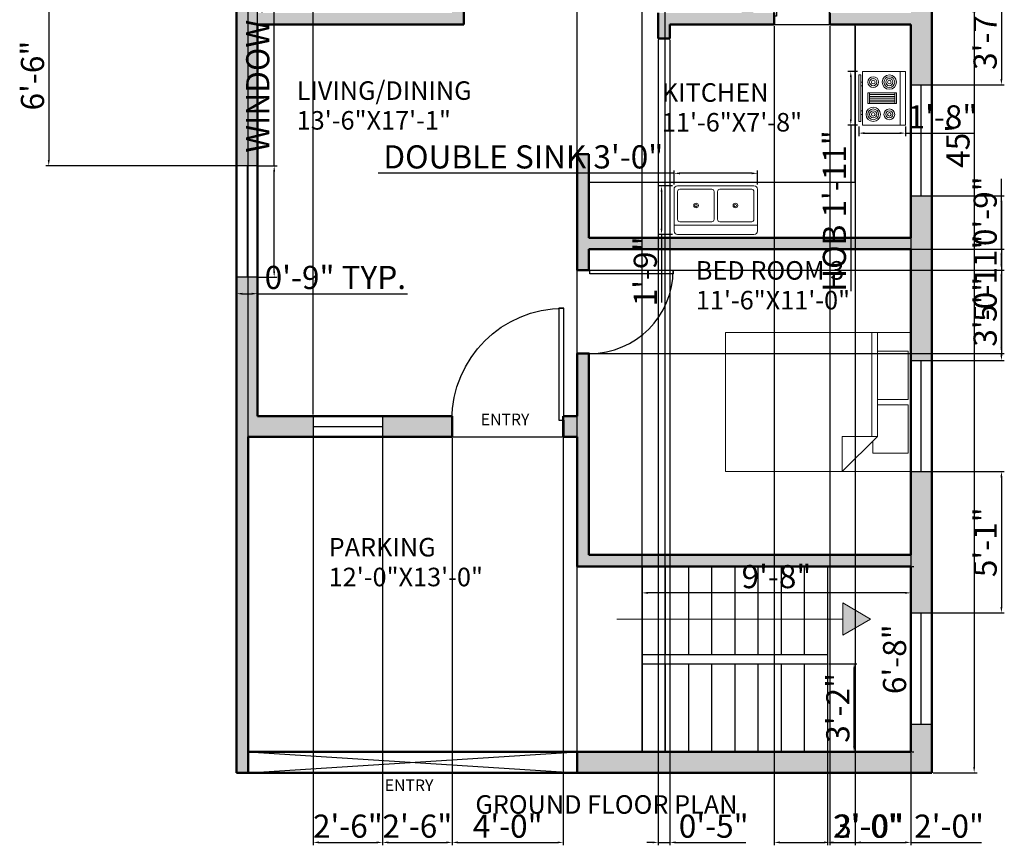
# Model space of a CAD drawing. Units: inches. Extents: x 3560 to 3985, y 1331 to 2044.
# Tile 1 of 2: x 3560 to 3985, y 1331 to 1688. Entities that reach past the tile are written whole.
import ezdxf

# ---------------------------------------------------------------- set-up
doc = ezdxf.new("R2010")
doc.units = ezdxf.units.IN
for name, color, linetype, lineweight in [('A-ANNO-DIMS', 5, 'Continuous', 18), ('A-ANNO-SYMB', 3, 'Continuous', 18), ('A-ANNO-TEXT', 2, 'Continuous', 25), ('A-AREA-IDEN', 3, 'Continuous', 25), ('A-EQPM', 8, 'Continuous', 18), ('A-FLOR-CASE', 8, 'Continuous', 25), ('A-FLOR-FIXT', 9, 'Continuous', 18), ('A-FURN', 8, 'Continuous', 18), ('A-WALL-PATT', 7, 'Continuous', 13), ('DOOR', 6, 'Continuous', 25), ('STAIRS', 1, 'Continuous', 25), ('WALL', 52, 'Continuous', 50), ('WINDOW', 4, 'Continuous', 25)]:
    doc.layers.add(name, color=color, linetype=linetype, lineweight=lineweight)
doc.styles.get("Standard").update_dxf_attribs({"font": 'arial.ttf'})
doc.dimstyles.new('ISO-25', dxfattribs={"dimtxt": 10, "dimasz": 2.5, "dimexe": 1.25, "dimexo": 0.625, "dimtad": 1, "dimdec": 1, "dimlunit": 3, "dimtxsty": 'Standard', "dimcen": 2.5, "dimadec": 0, "dimazin": 0, "dimtfac": 1, "dimtdec": 1, "dimtmove": 0, "dimatfit": 3, "dimfxl": 1, "dimarcsym": 0})

# ---------------------------------------------------------------- blocks, each defined once
blk = doc.blocks.new('*D1')
at = {"layer": 'A-ANNO-DIMS', "color": 0, "lineweight": -2, "transparency": 16777216}
for p, q in [((3828.42, 1450.94), (3828.42, 1438.95)), ((3944.42, 1450.94), (3944.42, 1438.95)), ((3941.92, 1440.2), (3830.92, 1440.2))]:
    blk.add_line(p, q, dxfattribs=at)
at = {"layer": 'A-ANNO-DIMS', "color": 0, "transparency": 16777216}
for points in [[(3830.92, 1440.62), (3830.92, 1439.78), (3828.42, 1440.2)], [(3941.92, 1440.62), (3941.92, 1439.78), (3944.42, 1440.2)]]:
    blk.add_solid(points, dxfattribs=at)
at = {"layer": 'Defpoints', "color": 0, "transparency": 16777216}
for p in [(3828.42, 1451.56), (3944.42, 1451.56), (3828.42, 1440.2)]:
    blk.add_point(p, dxfattribs=at)
at = {"layer": 'A-ANNO-DIMS', "color": 0, "transparency": 16777216, "insert": (3886.42, 1445.93), "char_height": 10, "attachment_point": 5}
blk.add_mtext('9\'-8"', dxfattribs=at)
blk = doc.blocks.new('*D2')
at = {"layer": 'A-ANNO-DIMS', "color": 0, "lineweight": -2, "transparency": 16777216}
for p, q in [((3945.04, 1451.56), (3945.67, 1451.56)), ((3944.42, 1449.06), (3944.42, 1374.06)), ((3945.04, 1371.56), (3945.67, 1371.56))]:
    blk.add_line(p, q, dxfattribs=at)
at = {"layer": 'A-ANNO-DIMS', "color": 0, "transparency": 16777216}
for points in [[(3944, 1449.06), (3944.83, 1449.06), (3944.42, 1451.56)], [(3944, 1374.06), (3944.83, 1374.06), (3944.42, 1371.56)]]:
    blk.add_solid(points, dxfattribs=at)
at = {"layer": 'Defpoints', "color": 0, "transparency": 16777216}
for p in [(3944.42, 1451.56), (3944.42, 1371.56), (3944.42, 1371.56)]:
    blk.add_point(p, dxfattribs=at)
at = {"layer": 'A-ANNO-DIMS', "color": 0, "transparency": 16777216, "insert": (3938.69, 1411.56), "char_height": 10, "attachment_point": 5, "rotation": 90}
blk.add_mtext('6\'-8"', dxfattribs=at)
blk = doc.blocks.new('*D3')
at = {"layer": 'A-ANNO-DIMS', "color": 0, "lineweight": -2, "transparency": 16777216}
for p, q in [((3909.04, 1409.56), (3921.18, 1409.56)), ((3919.93, 1374.06), (3919.93, 1407.06)), ((3909.04, 1371.56), (3921.18, 1371.56))]:
    blk.add_line(p, q, dxfattribs=at)
at = {"layer": 'A-ANNO-DIMS', "color": 0, "transparency": 16777216}
for points in [[(3919.52, 1407.06), (3920.35, 1407.06), (3919.93, 1409.56)], [(3919.52, 1374.06), (3920.35, 1374.06), (3919.93, 1371.56)]]:
    blk.add_solid(points, dxfattribs=at)
at = {"layer": 'Defpoints', "color": 0, "transparency": 16777216}
for p in [(3908.42, 1409.56), (3919.93, 1409.56), (3908.42, 1371.56)]:
    blk.add_point(p, dxfattribs=at)
at = {"layer": 'A-ANNO-DIMS', "color": 0, "transparency": 16777216, "insert": (3914.2, 1390.56), "char_height": 10, "attachment_point": 5, "rotation": 90}
blk.add_mtext('3\'-2"', dxfattribs=at)
blk = doc.blocks.new('*U5')
for p, q in [((0, 0), (0, -6)), ((40, 0), (40, -6))]:
    blk.add_line(p, q)
blk.add_lwpolyline([(0, 0), (0, 40), (1.75, 40), (1.75, 0)], close=True)
blk.add_arc((0, 0), 40, 0, 90)
blk = doc.blocks.new('Range-Oven - 30 in top')
for p, q in [((0, -3), (30, -3)), ((12, -6), (18, -6)), ((13, -20), (13, -6)), ((14, -6), (14, -20)), ((15, -20), (15, -6)), ((16, -6), (16, -20)), ((17, -20), (17, -6)), ((18, -20), (12, -20)), ((6, -24), (6, -25)), ((8, -25), (8, -24)), ((22, -25), (22, -24)), ((24, -24), (24, -25))]:
    blk.add_line(p, q)
for points in [[(0, -24), (0, 0), (30, 0), (30, -24)], [(12, -21), (12, -5), (18, -5), (18, -21)], [(2, -26), (2, -25), (28, -25), (28, -26)]]:
    blk.add_lwpolyline(points, close=True)
for centre, radius in [((6, -9), 4), ((6, -9), 3), ((6, -9), 2), ((6, -9), 1), ((24, -9), 3), ((24, -9), 2), ((24, -9), 1), ((6, -18), 3), ((6, -18), 2), ((24, -18), 4), ((24, -18), 3), ((24, -18), 2), ((6, -18), 1), ((24, -18), 1)]:
    blk.add_circle(centre, radius)
blk = doc.blocks.new('Sink-double - 36 in top')
for p, q in [((-18, -4), (18, -4)), ((-0.75, -18.5), (-0.75, -6.5)), ((0.75, -6.5), (0.75, -18.5))]:
    blk.add_line(p, q)
for points in [[(-16.5, 0), (16.5, 0)], [(-18, -19.5), (-18, -1.5)], [(18, -1.5), (18, -19.5)], [(-16.5, -18.5), (-16.5, -6.5)], [(-15.5, -5.5), (-1.75, -5.5)], [(1.75, -5.5), (15.5, -5.5)], [(16.5, -6.5), (16.5, -18.5)], [(16.5, -21), (-16.5, -21)], [(-1.75, -19.5), (-15.5, -19.5)], [(15.5, -19.5), (1.75, -19.5)]]:
    blk.add_lwpolyline(points)
for centre, radius in [((-8.5, -12.5), 1), ((-8.5, -12.5), 0.5), ((8.5, -12.5), 1), ((8.5, -12.5), 0.5)]:
    blk.add_circle(centre, radius)
for centre, radius, start, end in [((-16.5, -1.5), 1.5, 90, 180), ((16.5, -1.5), 1.5, 0, 90), ((-15.5, -6.5), 1, 90, 180), ((-1.75, -6.5), 1, 0, 90), ((1.75, -6.5), 1, 90, 180), ((15.5, -6.5), 1, 0, 90), ((-16.5, -19.5), 1.5, 180, 270), ((-15.5, -18.5), 1, 180, 270), ((-1.75, -18.5), 1, 270, 0), ((1.75, -18.5), 1, 180, 270), ((15.5, -18.5), 1, 270, 0), ((16.5, -19.5), 1.5, 270, 0)]:
    blk.add_arc(centre, radius, start, end)
blk = doc.blocks.new('Bed - Queen')
for p, q in [((0, -80.00003), (0, 0)), ((0, 0), (59.99999, 0)), ((59.99999, 0), (59.99999, -80.00003)), ((7.99999, -1.2), (28.79998, -1.2)), ((7.99999, -14.4), (7.99999, -1.2)), ((28.79998, -1.2), (28.79998, -14.4)), ((31.19999, -1.2), (51.99999, -1.2)), ((31.19999, -14.4), (31.19999, -1.2)), ((51.99999, -1.2), (51.99999, -16.4)), ((0, -14.4), (44.8, -14.4)), ((44.8, -16.8), (0, -16.8)), ((59.99999, -29.6), (44.8, -14.4)), ((44.8, -14.4), (44.8, -29.6)), ((51.99999, -16.4), (46.79936, -16.4)), ((44.8, -29.6), (59.99999, -29.6)), ((59.99999, -80.00003), (0, -80.00003))]:
    blk.add_line(p, q)
blk = doc.blocks.new('*D12')
at = {"layer": 'A-ANNO-DIMS', "color": 0, "lineweight": -2, "transparency": 16777216}
for p, q in [((3954.04, 1902.56), (3973, 1902.56)), ((3971.75, 1900.06), (3971.75, 1365.06)), ((3954.04, 1362.56), (3973, 1362.56))]:
    blk.add_line(p, q, dxfattribs=at)
at = {"layer": 'A-ANNO-DIMS', "color": 0, "transparency": 16777216}
for points in [[(3971.33, 1900.06), (3972.16, 1900.06), (3971.75, 1902.56)], [(3971.33, 1365.06), (3972.16, 1365.06), (3971.75, 1362.56)]]:
    blk.add_solid(points, dxfattribs=at)
at = {"layer": 'Defpoints', "color": 0, "transparency": 16777216}
for p in [(3953.42, 1902.56), (3953.42, 1362.56), (3971.75, 1362.56)]:
    blk.add_point(p, dxfattribs=at)
at = {"layer": 'A-ANNO-DIMS', "color": 0, "transparency": 16777216, "insert": (3966.04, 1633.18), "char_height": 10, "attachment_point": 5, "rotation": 90}
blk.add_mtext("45'", dxfattribs=at)
blk = doc.blocks.new('WIN-48IN')
for p, q in [((9, 48), (0, 48)), ((4.5, 48), (4.5, 0)), ((9, 0), (0, 0))]:
    blk.add_line(p, q)
blk = doc.blocks.new('*D20')
at = {"layer": 'A-ANNO-DIMS', "color": 0, "lineweight": -2, "transparency": 16777216}
for p, q in [((3669.62, 1624.56), (3669.62, 1754.85)), ((3663.04, 1624.56), (3670.87, 1624.56)), ((3669.62, 1579.06), (3669.62, 1622.06)), ((3663.04, 1576.56), (3670.87, 1576.56))]:
    blk.add_line(p, q, dxfattribs=at)
at = {"layer": 'A-ANNO-DIMS', "color": 0, "transparency": 16777216}
for points in [[(3669.2, 1622.06), (3670.03, 1622.06), (3669.62, 1624.56)], [(3669.2, 1579.06), (3670.03, 1579.06), (3669.62, 1576.56)]]:
    blk.add_solid(points, dxfattribs=at)
at = {"layer": 'Defpoints', "color": 0, "transparency": 16777216}
for p in [(3662.42, 1624.56), (3669.62, 1624.56), (3662.42, 1576.56)]:
    blk.add_point(p, dxfattribs=at)
at = {"layer": 'A-ANNO-DIMS', "color": 0, "transparency": 16777216, "insert": (3663.82, 1690.96), "char_height": 10, "attachment_point": 5, "rotation": 90}
blk.add_mtext('WINDOW 4\'-0" TYP.', dxfattribs=at)
blk = doc.blocks.new('*D21')
at = {"layer": 'A-ANNO-DIMS', "color": 0, "lineweight": -2, "transparency": 16777216}
for p, q in [((3653.42, 1575.94), (3653.42, 1568.11)), ((3662.42, 1575.94), (3662.42, 1568.11)), ((3655.92, 1569.36), (3659.92, 1569.36)), ((3662.42, 1569.36), (3727.12, 1569.36))]:
    blk.add_line(p, q, dxfattribs=at)
at = {"layer": 'A-ANNO-DIMS', "color": 0, "transparency": 16777216}
for points in [[(3655.92, 1569.78), (3655.92, 1568.95), (3653.42, 1569.36)], [(3659.92, 1569.78), (3659.92, 1568.95), (3662.42, 1569.36)]]:
    blk.add_solid(points, dxfattribs=at)
at = {"layer": 'Defpoints', "color": 0, "transparency": 16777216}
for p in [(3653.42, 1576.56), (3662.42, 1576.56), (3662.42, 1569.36)]:
    blk.add_point(p, dxfattribs=at)
at = {"layer": 'A-ANNO-DIMS', "color": 0, "transparency": 16777216, "insert": (3696.02, 1575.09), "char_height": 10, "attachment_point": 5}
blk.add_mtext('0\'-9" TYP.', dxfattribs=at)
blk = doc.blocks.new('*D24')
at = {"layer": 'A-ANNO-DIMS', "color": 0, "lineweight": -2, "transparency": 16777216}
for p, q in [((3921.37, 1665.36), (3917.26, 1665.36)), ((3918.51, 1662.86), (3918.51, 1644.66)), ((3921.37, 1642.16), (3917.26, 1642.16)), ((3918.51, 1642.16), (3918.51, 1570.44))]:
    blk.add_line(p, q, dxfattribs=at)
at = {"layer": 'A-ANNO-DIMS', "color": 0, "transparency": 16777216}
for points in [[(3918.1, 1662.86), (3918.93, 1662.86), (3918.51, 1665.36)], [(3918.1, 1644.66), (3918.93, 1644.66), (3918.51, 1642.16)]]:
    blk.add_solid(points, dxfattribs=at)
at = {"layer": 'Defpoints', "color": 0, "transparency": 16777216}
for p in [(3921.99, 1665.36), (3918.51, 1642.16), (3921.99, 1642.16)]:
    blk.add_point(p, dxfattribs=at)
at = {"layer": 'A-ANNO-DIMS', "color": 0, "transparency": 16777216, "insert": (3912.72, 1605.05), "char_height": 10, "attachment_point": 5, "rotation": 90}
blk.add_mtext('HOB 1\'-11"', dxfattribs=at)
blk = doc.blocks.new('*D25')
at = {"layer": 'A-ANNO-DIMS', "color": 0, "lineweight": -2, "transparency": 16777216}
for p, q in [((3921.99, 1641.54), (3921.99, 1637.43)), ((3942.1, 1641.54), (3942.1, 1637.43)), ((3924.49, 1638.68), (3939.6, 1638.68)), ((3942.1, 1638.68), (3971.49, 1638.68))]:
    blk.add_line(p, q, dxfattribs=at)
at = {"layer": 'A-ANNO-DIMS', "color": 0, "transparency": 16777216}
for points in [[(3924.49, 1639.1), (3924.49, 1638.26), (3921.99, 1638.68)], [(3939.6, 1639.1), (3939.6, 1638.26), (3942.1, 1638.68)]]:
    blk.add_solid(points, dxfattribs=at)
at = {"layer": 'Defpoints', "color": 0, "transparency": 16777216}
for p in [(3921.99, 1642.16), (3942.1, 1642.16), (3942.1, 1638.68)]:
    blk.add_point(p, dxfattribs=at)
at = {"layer": 'A-ANNO-DIMS', "color": 0, "transparency": 16777216, "insert": (3958.04, 1644.41), "char_height": 10, "attachment_point": 5}
blk.add_mtext('1\'-8"', dxfattribs=at)
blk = doc.blocks.new('*D26')
at = {"layer": 'A-ANNO-DIMS', "color": 0, "lineweight": -2, "transparency": 16777216}
for p, q in [((3842.22, 1621.34), (3714.57, 1621.34)), ((3842.22, 1616.56), (3842.22, 1622.59)), ((3875.72, 1621.34), (3844.72, 1621.34)), ((3878.22, 1616.56), (3878.22, 1622.59))]:
    blk.add_line(p, q, dxfattribs=at)
at = {"layer": 'A-ANNO-DIMS', "color": 0, "transparency": 16777216}
for points in [[(3844.72, 1621.75), (3844.72, 1620.92), (3842.22, 1621.34)], [(3875.72, 1621.75), (3875.72, 1620.92), (3878.22, 1621.34)]]:
    blk.add_solid(points, dxfattribs=at)
at = {"layer": 'Defpoints', "color": 0, "transparency": 16777216}
for p in [(3842.22, 1621.34), (3842.22, 1615.94), (3878.22, 1615.94)]:
    blk.add_point(p, dxfattribs=at)
at = {"layer": 'A-ANNO-DIMS', "color": 0, "transparency": 16777216, "insert": (3777.15, 1627.14), "char_height": 10, "attachment_point": 5}
blk.add_mtext('DOUBLE SINK 3\'-0"', dxfattribs=at)
blk = doc.blocks.new('*D27')
at = {"layer": 'A-ANNO-DIMS', "color": 0, "lineweight": -2, "transparency": 16777216}
for p, q in [((3841.6, 1615.94), (3835.57, 1615.94)), ((3836.82, 1613.44), (3836.82, 1597.44)), ((3841.6, 1594.94), (3835.57, 1594.94)), ((3836.82, 1594.94), (3836.82, 1565.54))]:
    blk.add_line(p, q, dxfattribs=at)
at = {"layer": 'A-ANNO-DIMS', "color": 0, "transparency": 16777216}
for points in [[(3836.41, 1613.44), (3837.24, 1613.44), (3836.82, 1615.94)], [(3836.41, 1597.44), (3837.24, 1597.44), (3836.82, 1594.94)]]:
    blk.add_solid(points, dxfattribs=at)
at = {"layer": 'Defpoints', "color": 0, "transparency": 16777216}
for p in [(3842.22, 1615.94), (3836.82, 1594.94), (3842.22, 1594.94)]:
    blk.add_point(p, dxfattribs=at)
at = {"layer": 'A-ANNO-DIMS', "color": 0, "transparency": 16777216, "insert": (3831.09, 1578.99), "char_height": 10, "attachment_point": 5, "rotation": 90}
blk.add_mtext('1\'-9"', dxfattribs=at)
blk = doc.blocks.new('*D30')
at = {"layer": 'A-ANNO-DIMS', "color": 0, "lineweight": -2, "transparency": 16777216}
for p, q in [((3652.79, 1702.56), (3571.07, 1702.56)), ((3572.32, 1700.06), (3572.32, 1627.06)), ((3652.79, 1624.56), (3571.07, 1624.56))]:
    blk.add_line(p, q, dxfattribs=at)
at = {"layer": 'A-ANNO-DIMS', "color": 0, "transparency": 16777216}
for points in [[(3571.9, 1700.06), (3572.73, 1700.06), (3572.32, 1702.56)], [(3571.9, 1627.06), (3572.73, 1627.06), (3572.32, 1624.56)]]:
    blk.add_solid(points, dxfattribs=at)
at = {"layer": 'Defpoints', "color": 0, "transparency": 16777216}
for p in [(3653.42, 1702.56), (3572.32, 1624.56), (3653.42, 1624.56)]:
    blk.add_point(p, dxfattribs=at)
at = {"layer": 'A-ANNO-DIMS', "color": 0, "transparency": 16777216, "insert": (3566.59, 1663.56), "char_height": 10, "attachment_point": 5, "rotation": 90}
blk.add_mtext('6\'-6"', dxfattribs=at)
blk = doc.blocks.new('*D33')
at = {"layer": 'A-ANNO-DIMS', "color": 0, "lineweight": -2, "transparency": 16777216}
for p, q in [((3954.04, 1702.56), (3984.77, 1702.56)), ((3983.52, 1700.06), (3983.52, 1662.06)), ((3954.04, 1659.56), (3984.77, 1659.56))]:
    blk.add_line(p, q, dxfattribs=at)
at = {"layer": 'A-ANNO-DIMS', "color": 0, "transparency": 16777216}
for points in [[(3983.1, 1700.06), (3983.93, 1700.06), (3983.52, 1702.56)], [(3983.1, 1662.06), (3983.93, 1662.06), (3983.52, 1659.56)]]:
    blk.add_solid(points, dxfattribs=at)
at = {"layer": 'Defpoints', "color": 0, "transparency": 16777216}
for p in [(3953.42, 1702.56), (3953.42, 1659.56), (3983.52, 1659.56)]:
    blk.add_point(p, dxfattribs=at)
at = {"layer": 'A-ANNO-DIMS', "color": 0, "transparency": 16777216, "insert": (3977.78, 1681.06), "char_height": 10, "attachment_point": 5, "rotation": 90}
blk.add_mtext('3\'-7"', dxfattribs=at)
blk = doc.blocks.new('*D34')
at = {"layer": 'A-ANNO-DIMS', "color": 0, "lineweight": -2, "transparency": 16777216}
for p, q in [((3954.04, 1611.56), (3984.77, 1611.56)), ((3983.52, 1609.06), (3983.52, 1543.06)), ((3954.04, 1540.56), (3984.77, 1540.56))]:
    blk.add_line(p, q, dxfattribs=at)
at = {"layer": 'A-ANNO-DIMS', "color": 0, "transparency": 16777216}
for points in [[(3983.1, 1609.06), (3983.93, 1609.06), (3983.52, 1611.56)], [(3983.1, 1543.06), (3983.93, 1543.06), (3983.52, 1540.56)]]:
    blk.add_solid(points, dxfattribs=at)
at = {"layer": 'Defpoints', "color": 0, "transparency": 16777216}
for p in [(3953.42, 1611.56), (3953.42, 1540.56), (3983.52, 1540.56)]:
    blk.add_point(p, dxfattribs=at)
at = {"layer": 'A-ANNO-DIMS', "color": 0, "transparency": 16777216, "insert": (3977.79, 1576.06), "char_height": 10, "attachment_point": 5, "rotation": 90}
blk.add_mtext('5\'-11"', dxfattribs=at)
blk = doc.blocks.new('*D35')
at = {"layer": 'A-ANNO-DIMS', "color": 0, "lineweight": -2, "transparency": 16777216}
for p, q in [((3954.04, 1492.56), (3984.77, 1492.56)), ((3983.52, 1490.06), (3983.52, 1434.06)), ((3954.04, 1431.56), (3984.77, 1431.56))]:
    blk.add_line(p, q, dxfattribs=at)
at = {"layer": 'A-ANNO-DIMS', "color": 0, "transparency": 16777216}
for points in [[(3983.1, 1490.06), (3983.93, 1490.06), (3983.52, 1492.56)], [(3983.1, 1434.06), (3983.93, 1434.06), (3983.52, 1431.56)]]:
    blk.add_solid(points, dxfattribs=at)
at = {"layer": 'Defpoints', "color": 0, "transparency": 16777216}
for p in [(3953.42, 1492.56), (3953.42, 1431.56), (3983.52, 1431.56)]:
    blk.add_point(p, dxfattribs=at)
at = {"layer": 'A-ANNO-DIMS', "color": 0, "transparency": 16777216, "insert": (3977.79, 1462.06), "char_height": 10, "attachment_point": 5, "rotation": 90}
blk.add_mtext('5\'-1"', dxfattribs=at)
blk = doc.blocks.new('*D36')
at = {"layer": 'A-ANNO-DIMS', "color": 0, "lineweight": -2, "transparency": 16777216}
for p, q in [((3662.42, 1517.19), (3662.42, 1933.91)), ((3686.42, 1517.19), (3686.42, 1933.91)), ((3664.92, 1932.66), (3683.92, 1932.66)), ((3686.42, 1932.66), (3716.92, 1932.66))]:
    blk.add_line(p, q, dxfattribs=at)
at = {"layer": 'A-ANNO-DIMS', "color": 0, "transparency": 16777216}
for points in [[(3664.92, 1933.08), (3664.92, 1932.25), (3662.42, 1932.66)], [(3683.92, 1933.08), (3683.92, 1932.25), (3686.42, 1932.66)]]:
    blk.add_solid(points, dxfattribs=at)
at = {"layer": 'Defpoints', "color": 0, "transparency": 16777216}
for p in [(3686.42, 1932.66), (3662.42, 1516.56), (3686.42, 1516.56)]:
    blk.add_point(p, dxfattribs=at)
at = {"layer": 'A-ANNO-DIMS', "color": 0, "transparency": 16777216, "insert": (3702.92, 1938.39), "char_height": 10, "attachment_point": 5}
blk.add_mtext('2\'-0"', dxfattribs=at)
blk = doc.blocks.new('*D37')
at = {"layer": 'A-ANNO-DIMS', "color": 0, "lineweight": -2, "transparency": 16777216}
for p, q in [((3686.42, 1506.94), (3686.42, 1331.21)), ((3716.42, 1506.94), (3716.42, 1331.21)), ((3688.92, 1332.46), (3713.92, 1332.46))]:
    blk.add_line(p, q, dxfattribs=at)
at = {"layer": 'A-ANNO-DIMS', "color": 0, "transparency": 16777216}
for points in [[(3688.92, 1332.88), (3688.92, 1332.05), (3686.42, 1332.46)], [(3713.92, 1332.88), (3713.92, 1332.05), (3716.42, 1332.46)]]:
    blk.add_solid(points, dxfattribs=at)
at = {"layer": 'Defpoints', "color": 0, "transparency": 16777216}
for p in [(3686.42, 1507.56), (3716.42, 1507.56), (3716.42, 1332.46)]:
    blk.add_point(p, dxfattribs=at)
at = {"layer": 'A-ANNO-DIMS', "color": 0, "transparency": 16777216, "insert": (3701.42, 1338.19), "char_height": 10, "attachment_point": 5}
blk.add_mtext('2\'-6"', dxfattribs=at)
blk = doc.blocks.new('*D38')
at = {"layer": 'A-ANNO-DIMS', "color": 0, "lineweight": -2, "transparency": 16777216}
for p, q in [((3716.42, 1506.94), (3716.42, 1331.21)), ((3746.42, 1506.94), (3746.42, 1331.21)), ((3718.92, 1332.46), (3743.92, 1332.46))]:
    blk.add_line(p, q, dxfattribs=at)
at = {"layer": 'A-ANNO-DIMS', "color": 0, "transparency": 16777216}
for points in [[(3718.92, 1332.88), (3718.92, 1332.05), (3716.42, 1332.46)], [(3743.92, 1332.88), (3743.92, 1332.05), (3746.42, 1332.46)]]:
    blk.add_solid(points, dxfattribs=at)
at = {"layer": 'Defpoints', "color": 0, "transparency": 16777216}
for p in [(3716.42, 1507.56), (3746.42, 1507.56), (3746.42, 1332.46)]:
    blk.add_point(p, dxfattribs=at)
at = {"layer": 'A-ANNO-DIMS', "color": 0, "transparency": 16777216, "insert": (3731.42, 1338.19), "char_height": 10, "attachment_point": 5}
blk.add_mtext('2\'-6"', dxfattribs=at)
blk = doc.blocks.new('*D39')
at = {"layer": 'A-ANNO-DIMS', "color": 0, "lineweight": -2, "transparency": 16777216}
for p, q in [((3746.42, 1506.94), (3746.42, 1331.21)), ((3794.42, 1506.94), (3794.42, 1331.21)), ((3748.92, 1332.46), (3791.92, 1332.46))]:
    blk.add_line(p, q, dxfattribs=at)
at = {"layer": 'A-ANNO-DIMS', "color": 0, "transparency": 16777216}
for points in [[(3748.92, 1332.88), (3748.92, 1332.05), (3746.42, 1332.46)], [(3791.92, 1332.88), (3791.92, 1332.05), (3794.42, 1332.46)]]:
    blk.add_solid(points, dxfattribs=at)
at = {"layer": 'Defpoints', "color": 0, "transparency": 16777216}
for p in [(3746.42, 1507.56), (3794.42, 1507.56), (3794.42, 1332.46)]:
    blk.add_point(p, dxfattribs=at)
at = {"layer": 'A-ANNO-DIMS', "color": 0, "transparency": 16777216, "insert": (3770.42, 1338.19), "char_height": 10, "attachment_point": 5}
blk.add_mtext('4\'-0"', dxfattribs=at)
blk = doc.blocks.new('*D44')
at = {"layer": 'A-ANNO-DIMS', "color": 0, "lineweight": -2, "transparency": 16777216}
for p, q in [((3885.42, 1684.94), (3885.42, 1331.21)), ((3909.42, 1684.94), (3909.42, 1331.21)), ((3887.92, 1332.46), (3906.92, 1332.46)), ((3909.42, 1332.46), (3939.92, 1332.46))]:
    blk.add_line(p, q, dxfattribs=at)
at = {"layer": 'A-ANNO-DIMS', "color": 0, "transparency": 16777216}
for points in [[(3887.92, 1332.88), (3887.92, 1332.05), (3885.42, 1332.46)], [(3906.92, 1332.88), (3906.92, 1332.05), (3909.42, 1332.46)]]:
    blk.add_solid(points, dxfattribs=at)
at = {"layer": 'Defpoints', "color": 0, "transparency": 16777216}
for p in [(3885.42, 1685.56), (3909.42, 1685.56), (3909.42, 1332.46)]:
    blk.add_point(p, dxfattribs=at)
at = {"layer": 'A-ANNO-DIMS', "color": 0, "transparency": 16777216, "insert": (3925.92, 1338.19), "char_height": 10, "attachment_point": 5}
blk.add_mtext('2\'-0"', dxfattribs=at)
blk = doc.blocks.new('*D46')
at = {"layer": 'A-ANNO-DIMS', "color": 0, "lineweight": -2, "transparency": 16777216}
for p, q in [((3920.42, 1684.94), (3920.42, 1331.21)), ((3944.42, 1684.94), (3944.42, 1331.21)), ((3922.92, 1332.46), (3941.92, 1332.46)), ((3944.42, 1332.46), (3974.92, 1332.46))]:
    blk.add_line(p, q, dxfattribs=at)
at = {"layer": 'A-ANNO-DIMS', "color": 0, "transparency": 16777216}
for points in [[(3922.92, 1332.88), (3922.92, 1332.05), (3920.42, 1332.46)], [(3941.92, 1332.88), (3941.92, 1332.05), (3944.42, 1332.46)]]:
    blk.add_solid(points, dxfattribs=at)
at = {"layer": 'Defpoints', "color": 0, "transparency": 16777216}
for p in [(3920.42, 1685.56), (3944.42, 1685.56), (3944.42, 1332.46)]:
    blk.add_point(p, dxfattribs=at)
at = {"layer": 'A-ANNO-DIMS', "color": 0, "transparency": 16777216, "insert": (3960.92, 1338.19), "char_height": 10, "attachment_point": 5}
blk.add_mtext('2\'-0"', dxfattribs=at)
blk = doc.blocks.new('*D49')
at = {"layer": 'A-ANNO-DIMS', "color": 0, "lineweight": -2, "transparency": 16777216}
for p, q in [((3806.04, 1579.56), (3984.77, 1579.56)), ((3983.52, 1546.06), (3983.52, 1577.06)), ((3806.04, 1543.56), (3984.77, 1543.56))]:
    blk.add_line(p, q, dxfattribs=at)
at = {"layer": 'A-ANNO-DIMS', "color": 0, "transparency": 16777216}
for points in [[(3983.1, 1577.06), (3983.93, 1577.06), (3983.52, 1579.56)], [(3983.1, 1546.06), (3983.93, 1546.06), (3983.52, 1543.56)]]:
    blk.add_solid(points, dxfattribs=at)
at = {"layer": 'Defpoints', "color": 0, "transparency": 16777216}
for p in [(3805.42, 1579.56), (3983.52, 1579.56), (3805.42, 1543.56)]:
    blk.add_point(p, dxfattribs=at)
at = {"layer": 'A-ANNO-DIMS', "color": 0, "transparency": 16777216, "insert": (3977.78, 1561.56), "char_height": 10, "attachment_point": 5, "rotation": 90}
blk.add_mtext('3\'-0"', dxfattribs=at)
blk = doc.blocks.new('*D50')
at = {"layer": 'A-ANNO-DIMS', "color": 0, "lineweight": -2, "transparency": 16777216}
for p, q in [((3983.52, 1588.56), (3983.52, 1618.9)), ((3806.04, 1588.56), (3984.77, 1588.56)), ((3983.52, 1582.06), (3983.52, 1586.06)), ((3806.04, 1579.56), (3984.77, 1579.56))]:
    blk.add_line(p, q, dxfattribs=at)
at = {"layer": 'A-ANNO-DIMS', "color": 0, "transparency": 16777216}
for points in [[(3983.1, 1586.06), (3983.93, 1586.06), (3983.52, 1588.56)], [(3983.1, 1582.06), (3983.93, 1582.06), (3983.52, 1579.56)]]:
    blk.add_solid(points, dxfattribs=at)
at = {"layer": 'Defpoints', "color": 0, "transparency": 16777216}
for p in [(3805.42, 1588.56), (3983.52, 1588.56), (3805.42, 1579.56)]:
    blk.add_point(p, dxfattribs=at)
at = {"layer": 'A-ANNO-DIMS', "color": 0, "transparency": 16777216, "insert": (3977.79, 1604.98), "char_height": 10, "attachment_point": 5, "rotation": 90}
blk.add_mtext('0\'-9"', dxfattribs=at)
blk = doc.blocks.new('*D51')
at = {"layer": 'A-ANNO-DIMS', "color": 0, "lineweight": -2, "transparency": 16777216}
for p, q in [((3835.42, 1678.94), (3835.42, 1331.21)), ((3840.42, 1678.94), (3840.42, 1331.21)), ((3832.92, 1332.46), (3830.42, 1332.46)), ((3835.42, 1332.46), (3840.42, 1332.46)), ((3842.92, 1332.46), (3873.25, 1332.46))]:
    blk.add_line(p, q, dxfattribs=at)
at = {"layer": 'A-ANNO-DIMS', "color": 0, "transparency": 16777216}
for points in [[(3832.92, 1332.88), (3832.92, 1332.05), (3835.42, 1332.46)], [(3842.92, 1332.88), (3842.92, 1332.05), (3840.42, 1332.46)]]:
    blk.add_solid(points, dxfattribs=at)
at = {"layer": 'Defpoints', "color": 0, "transparency": 16777216}
for p in [(3835.42, 1679.56), (3840.42, 1679.56), (3840.42, 1332.46)]:
    blk.add_point(p, dxfattribs=at)
at = {"layer": 'A-ANNO-DIMS', "color": 0, "transparency": 16777216, "insert": (3859.33, 1338.19), "char_height": 10, "attachment_point": 5}
blk.add_mtext('0\'-5"', dxfattribs=at)
blk = doc.blocks.new('*D52')
at = {"layer": 'A-ANNO-DIMS', "color": 0, "lineweight": -2, "transparency": 16777216}
for p, q in [((3658.42, 1372.19), (3658.42, 1933.91)), ((3800.42, 1372.19), (3800.42, 1933.91)), ((3660.92, 1932.66), (3797.92, 1932.66))]:
    blk.add_line(p, q, dxfattribs=at)
at = {"layer": 'A-ANNO-DIMS', "color": 0, "transparency": 16777216}
for points in [[(3660.92, 1933.08), (3660.92, 1932.25), (3658.42, 1932.66)], [(3797.92, 1933.08), (3797.92, 1932.25), (3800.42, 1932.66)]]:
    blk.add_solid(points, dxfattribs=at)
at = {"layer": 'Defpoints', "color": 0, "transparency": 16777216}
for p in [(3800.42, 1932.66), (3658.42, 1371.56), (3800.42, 1371.56)]:
    blk.add_point(p, dxfattribs=at)
at = {"layer": 'A-ANNO-DIMS', "color": 0, "transparency": 16777216, "insert": (3729.42, 1938.39), "char_height": 10, "attachment_point": 5}
blk.add_mtext('11\'-10"', dxfattribs=at)
blk = doc.blocks.new('*D53')
at = {"layer": 'A-ANNO-DIMS', "color": 0, "lineweight": -2, "transparency": 16777216}
for p, q in [((3828.42, 1372.19), (3828.42, 1933.91)), ((3838.42, 1372.19), (3838.42, 1933.91)), ((3830.92, 1932.66), (3835.92, 1932.66)), ((3838.42, 1932.66), (3876.52, 1932.66))]:
    blk.add_line(p, q, dxfattribs=at)
at = {"layer": 'A-ANNO-DIMS', "color": 0, "transparency": 16777216}
for points in [[(3830.92, 1933.08), (3830.92, 1932.25), (3828.42, 1932.66)], [(3835.92, 1933.08), (3835.92, 1932.25), (3838.42, 1932.66)]]:
    blk.add_solid(points, dxfattribs=at)
at = {"layer": 'Defpoints', "color": 0, "transparency": 16777216}
for p in [(3838.42, 1932.66), (3828.42, 1371.56), (3838.42, 1371.56)]:
    blk.add_point(p, dxfattribs=at)
at = {"layer": 'A-ANNO-DIMS', "color": 0, "transparency": 16777216, "insert": (3858.72, 1938.39), "char_height": 10, "attachment_point": 5}
blk.add_mtext('0\'-10"', dxfattribs=at)
blk = doc.blocks.new('*D54')
at = {"layer": 'A-ANNO-DIMS', "color": 0, "lineweight": -2, "transparency": 16777216}
for p, q in [((3908.42, 1450.94), (3908.42, 1331.21)), ((3944.42, 1450.94), (3944.42, 1331.21)), ((3910.92, 1332.46), (3941.92, 1332.46))]:
    blk.add_line(p, q, dxfattribs=at)
at = {"layer": 'A-ANNO-DIMS', "color": 0, "transparency": 16777216}
for points in [[(3910.92, 1332.88), (3910.92, 1332.05), (3908.42, 1332.46)], [(3941.92, 1332.88), (3941.92, 1332.05), (3944.42, 1332.46)]]:
    blk.add_solid(points, dxfattribs=at)
at = {"layer": 'Defpoints', "color": 0, "transparency": 16777216}
for p in [(3908.42, 1451.56), (3944.42, 1451.56), (3944.42, 1332.46)]:
    blk.add_point(p, dxfattribs=at)
at = {"layer": 'A-ANNO-DIMS', "color": 0, "transparency": 16777216, "insert": (3926.42, 1338.2), "char_height": 10, "attachment_point": 5}
blk.add_mtext('3\'-0"', dxfattribs=at)

msp = doc.modelspace()

# ---------------------------------------------------------------- hatches: boundary and pattern name
at = {"layer": 'A-ANNO-SYMB'}
h = msp.add_hatch(color=256, dxfattribs=at)
h.dxf.hatch_style = 1
h.paths.add_polyline_path([(3915.02, 1435.84), (3915.02, 1428.91), (3915.02, 1421.99), (3927.08, 1428.91)])
at = {"layer": 'A-WALL-PATT'}
h = msp.add_hatch(color=256, dxfattribs=at)
h.dxf.hatch_style = 1
h.paths.add_polyline_path([(3953.42, 1779.56), (3944.42, 1779.56), (3944.42, 1743.56), (3847.42, 1743.56), (3847.42, 1738.56), (3871.42, 1738.56), (3871.42, 1690.56), (3835.42, 1690.56), (3835.42, 1679.56), (3840.42, 1679.56), (3840.42, 1685.56), (3885.42, 1685.56), (3885.42, 1689.16), (3885.42, 1690.56), (3876.42, 1690.56), (3876.42, 1738.56), (3944.42, 1738.56), (3944.42, 1726.56), (3953.42, 1726.56)])
h = msp.add_hatch(color=256, dxfattribs=at)
h.dxf.hatch_style = 1
h.paths.add_polyline_path([(3662.42, 1685.56), (3751.42, 1685.56), (3751.42, 1696.56), (3747.82, 1696.56), (3746.42, 1696.56), (3746.42, 1690.56), (3662.42, 1690.56), (3662.42, 1702.56), (3653.42, 1702.56), (3653.42, 1624.56), (3662.42, 1624.56)])
h = msp.add_hatch(color=256, dxfattribs=at)
h.dxf.hatch_style = 1
h.paths.add_polyline_path([(3953.42, 1702.56), (3944.42, 1702.56), (3944.42, 1690.56), (3909.42, 1690.56), (3909.42, 1685.56), (3944.42, 1685.56), (3944.42, 1659.56), (3953.42, 1659.56)])
h = msp.add_hatch(color=256, dxfattribs=at)
h.dxf.hatch_style = 1
h.paths.add_polyline_path([(3953.42, 1611.56), (3944.42, 1611.56), (3944.42, 1593.56), (3805.42, 1593.56), (3805.42, 1629.56), (3800.42, 1629.56), (3800.42, 1579.56), (3805.42, 1579.56), (3805.42, 1588.56), (3944.42, 1588.56), (3944.42, 1540.56), (3953.42, 1540.56)])
h = msp.add_hatch(color=256, dxfattribs=at)
h.dxf.hatch_style = 1
h.paths.add_polyline_path([(3686.42, 1516.56), (3662.42, 1516.56), (3662.42, 1576.56), (3653.42, 1576.56), (3653.42, 1362.56), (3658.42, 1362.56), (3658.42, 1507.56), (3686.42, 1507.56)])
h = msp.add_hatch(color=256, dxfattribs=at)
h.dxf.hatch_style = 1
h.paths.add_polyline_path([(3953.42, 1492.56), (3944.42, 1492.56), (3944.42, 1456.56), (3805.42, 1456.56), (3805.42, 1543.56), (3800.42, 1543.56), (3800.42, 1516.56), (3794.62, 1516.56), (3794.62, 1514.81), (3794.62, 1507.56), (3800.42, 1507.56), (3800.42, 1451.56), (3944.42, 1451.56), (3944.42, 1431.56), (3953.42, 1431.56)])
h = msp.add_hatch(color=256, dxfattribs=at)
h.dxf.hatch_style = 1
h.paths.add_polyline_path([(3746.33, 1514.81, -0.009094), (3746.36, 1516.56), (3716.42, 1516.56), (3716.42, 1507.56), (3746.33, 1507.56)])
h = msp.add_hatch(color=256, dxfattribs=at)
h.dxf.hatch_style = 1
h.paths.add_polyline_path([(3953.42, 1383.56), (3944.42, 1383.56), (3944.42, 1371.56), (3800.42, 1371.56), (3800.42, 1362.56), (3953.42, 1362.56)])

# ---------------------------------------------------------------- linework, layer by layer
at = {"layer": 'A-ANNO-SYMB'}
for p, q in [((3915.02, 1428.91), (3915.02, 1435.84)), ((3915.02, 1435.84), (3927.08, 1428.91)), ((3817.55, 1428.91), (3915.02, 1428.91)), ((3915.02, 1428.91), (3915.02, 1421.99)), ((3915.02, 1421.99), (3927.08, 1428.91))]:
    msp.add_line(p, q, dxfattribs=at)
at = {"layer": 'A-FLOR-CASE'}
for p, q in [((3920.42, 1617.56), (3920.42, 1685.56)), ((3805.42, 1617.56), (3920.42, 1617.56))]:
    msp.add_line(p, q, dxfattribs=at)
at = {"layer": 'DOOR'}
for p, q in [((3885.42, 1685.56), (3909.42, 1685.56)), ((3800.42, 1543.56), (3800.42, 1579.56)), ((3746.42, 1507.56), (3794.42, 1507.56)), ((3658.42, 1362.56), (3800.42, 1371.56)), ((3658.42, 1371.56), (3800.42, 1362.56))]:
    msp.add_line(p, q, dxfattribs=at)
at = {"layer": 'STAIRS'}
for p, q in [((3828.42, 1451.56), (3828.42, 1371.56)), ((3838.42, 1451.56), (3838.42, 1413.56)), ((3848.42, 1451.56), (3848.42, 1413.56)), ((3858.42, 1451.56), (3858.42, 1413.56)), ((3868.42, 1451.56), (3868.42, 1413.56)), ((3878.42, 1451.56), (3878.42, 1413.56)), ((3888.42, 1451.56), (3888.42, 1413.56)), ((3898.42, 1451.56), (3898.42, 1413.56)), ((3908.42, 1451.56), (3908.42, 1371.56)), ((3828.42, 1413.56), (3908.42, 1413.56)), ((3828.42, 1409.56), (3908.42, 1409.56)), ((3838.42, 1409.56), (3838.42, 1371.56)), ((3848.42, 1409.56), (3848.42, 1371.56)), ((3858.42, 1409.56), (3858.42, 1371.56)), ((3868.42, 1409.56), (3868.42, 1371.56)), ((3878.42, 1409.56), (3878.42, 1371.56)), ((3888.42, 1409.56), (3888.42, 1371.56)), ((3898.42, 1409.56), (3898.42, 1371.56))]:
    msp.add_line(p, q, dxfattribs=at)
at = {"layer": 'WALL'}
for p, q in [((3653.42, 1902.56), (3653.42, 1362.56)), ((3953.42, 1902.56), (3953.42, 1362.56)), ((3751.42, 1696.56), (3751.42, 1685.56)), ((3835.42, 1690.56), (3835.42, 1679.56)), ((3885.42, 1690.56), (3885.42, 1685.56)), ((3909.42, 1690.56), (3909.42, 1685.56)), ((3662.42, 1685.56), (3751.42, 1685.56)), ((3662.42, 1685.56), (3662.42, 1516.56)), ((3840.42, 1685.56), (3885.42, 1685.56)), ((3840.42, 1685.56), (3840.42, 1679.56)), ((3909.42, 1685.56), (3944.42, 1685.56)), ((3944.42, 1685.56), (3944.42, 1593.56)), ((3835.42, 1679.56), (3840.42, 1679.56)), ((3800.42, 1629.56), (3800.42, 1579.56)), ((3805.42, 1629.56), (3800.42, 1629.56)), ((3805.42, 1629.56), (3805.42, 1593.56)), ((3805.42, 1593.56), (3944.42, 1593.56)), ((3805.42, 1588.56), (3944.42, 1588.56)), ((3805.42, 1588.56), (3805.42, 1579.56)), ((3944.42, 1588.56), (3944.42, 1456.56)), ((3805.42, 1579.56), (3800.42, 1579.56)), ((3805.42, 1543.56), (3800.42, 1543.56)), ((3800.42, 1543.56), (3800.42, 1516.56)), ((3805.42, 1543.56), (3805.42, 1456.56)), ((3662.42, 1516.56), (3746.42, 1516.56)), ((3746.42, 1516.56), (3746.42, 1507.56)), ((3794.42, 1516.56), (3794.42, 1507.56)), ((3794.42, 1516.56), (3800.42, 1516.56)), ((3658.42, 1507.56), (3658.42, 1362.56)), ((3658.42, 1507.56), (3746.42, 1507.56)), ((3794.42, 1507.56), (3800.42, 1507.56)), ((3800.42, 1507.56), (3800.42, 1451.56)), ((3805.42, 1456.56), (3944.42, 1456.56)), ((3800.42, 1451.56), (3944.42, 1451.56)), ((3944.42, 1451.56), (3944.42, 1371.56)), ((3658.42, 1371.56), (3944.42, 1371.56)), ((3800.42, 1371.56), (3800.42, 1362.56)), ((3653.42, 1362.56), (3953.42, 1362.56))]:
    msp.add_line(p, q, dxfattribs=at)
at = {"layer": 'WINDOW'}
for p, q in [((3686.42, 1516.56), (3686.42, 1507.56)), ((3716.42, 1516.56), (3716.42, 1507.56)), ((3686.42, 1512.06), (3716.42, 1512.06))]:
    msp.add_line(p, q, dxfattribs=at)

# ---------------------------------------------------------------- block references
at = {"layer": 'A-EQPM', "xscale": 0.7731837138245553, "yscale": 0.7731837138245553, "zscale": 0.7731837138245553, "rotation": 270}
msp.add_blockref('Range-Oven - 30 in top', (3942.1, 1665.36), dxfattribs=at)
at = {"layer": 'A-FLOR-FIXT', "rotation": 180}
msp.add_blockref('Sink-double - 36 in top', (3860.22, 1594.94), dxfattribs=at)
at = {"layer": 'A-FURN', "rotation": 270}
msp.add_blockref('Bed - Queen', (3944.42, 1552.56), dxfattribs=at)
at = {"layer": 'DOOR'}
for p, xscale, yscale, zscale in [((3885.42, 1689.16), 0.5999999999999819, 0.5999999999999819, 0.5999999999999819), ((3794.62, 1514.81), -1.207299289471573, 1.207299289471573, 1.207299289471573)]:
    msp.add_blockref('*U5', p, dxfattribs=dict(at, xscale=xscale, yscale=yscale, zscale=zscale))
at = {"layer": 'DOOR', "xscale": 0.8999999999999898, "yscale": 0.8999999999999898, "zscale": 0.8999999999999898, "rotation": 270}
msp.add_blockref('*U5', (3805.82, 1579.56), dxfattribs=at)
at = {"layer": 'WINDOW', "rotation": 180}
for p in [(3953.42, 1659.56), (3953.42, 1540.56), (3953.42, 1431.56)]:
    msp.add_blockref('WIN-48IN', p, dxfattribs=at)
at = {"layer": 'WINDOW'}
msp.add_blockref('WIN-48IN', (3653.42, 1576.56), dxfattribs=at)

# ---------------------------------------------------------------- texts
at = {"layer": 'A-ANNO-TEXT'}
for s, height, p in [('ENTRY', 5, (3758.79, 1512.6)), ('ENTRY', 5, (3717.34, 1354.67)), ('GROUND FLOOR PLAN', 8, (3756.45, 1344.84))]:
    msp.add_text(s, height=height, dxfattribs=at).set_placement(p)
at = {"layer": 'A-AREA-IDEN'}
for s, p in [('LIVING/DINING', (3679.32, 1653.06)), ('KITCHEN', (3836.96, 1652.24)), ('13\'-6"X17\'-1"', (3679.32, 1640.21)), ('11\'-6"X7\'-8"', (3836.96, 1639.39)), ('BED ROOM 3', (3851.61, 1575.43)), ('11\'-6"X11\'-0"', (3851.61, 1562.58)), ('PARKING', (3693.14, 1455.91)), ('12\'-0"X13\'-0"', (3693.14, 1443.05))]:
    msp.add_text(s, height=8, dxfattribs=at).set_placement(p)

# ---------------------------------------------------------------- dimensions: what is measured, and where the dimension line sits
at = {"layer": 'A-ANNO-DIMS'}
for base, p1, p2, override, picture, middle in [((3800.42, 1932.66), (3658.42, 1371.56), (3800.42, 1371.56), {"dimdec": 1, "dimlfac": 1, "dimrnd": 0, "dimzin": 1, "dimdsep": 46, "dimlunit": 4, "dimfrac": 2}, '*D52', (3729.42, 1938.39)), ((3686.42, 1932.66), (3662.42, 1516.56), (3686.42, 1516.56), {"dimdec": 1, "dimlfac": 1, "dimrnd": 0, "dimzin": 1, "dimdsep": 46, "dimlunit": 4, "dimfrac": 2}, '*D36', (3702.92, 1938.39)), ((3838.42, 1932.66), (3828.42, 1371.56), (3838.42, 1371.56), {"dimdec": 1, "dimlfac": 1, "dimrnd": 0, "dimzin": 1, "dimdsep": 46, "dimlunit": 4, "dimfrac": 2}, '*D53', (3858.72, 1938.39)), ((3909.42, 1332.46), (3885.42, 1685.56), (3909.42, 1685.56), {"dimdec": 1, "dimlfac": 1, "dimrnd": 0, "dimzin": 1, "dimdsep": 46, "dimlunit": 4, "dimfrac": 2}, '*D44', (3925.92, 1338.19)), ((3944.42, 1332.46), (3920.42, 1685.56), (3944.42, 1685.56), {"dimdec": 1, "dimlfac": 1, "dimrnd": 0, "dimzin": 1, "dimdsep": 46, "dimlunit": 4, "dimfrac": 2}, '*D46', (3960.92, 1338.19)), ((3840.42, 1332.46), (3835.42, 1679.56), (3840.42, 1679.56), {"dimdec": 1, "dimlfac": 1, "dimrnd": 0, "dimzin": 1, "dimdsep": 46, "dimlunit": 4, "dimfrac": 2}, '*D51', (3859.33, 1338.19)), ((3942.1, 1638.68), (3921.99, 1642.16), (3942.1, 1642.16), {"dimdec": 1, "dimlfac": 1, "dimrnd": 0, "dimzin": 1, "dimdsep": 46, "dimlunit": 4, "dimfrac": 2}, '*D25', (3958.04, 1644.41)), ((3716.42, 1332.46), (3686.42, 1507.56), (3716.42, 1507.56), {"dimdec": 1, "dimlfac": 1, "dimrnd": 0, "dimzin": 1, "dimdsep": 46, "dimlunit": 4, "dimfrac": 2}, '*D37', (3701.42, 1338.19)), ((3746.42, 1332.46), (3716.42, 1507.56), (3746.42, 1507.56), {"dimdec": 1, "dimlfac": 1, "dimrnd": 0, "dimzin": 1, "dimdsep": 46, "dimlunit": 4, "dimfrac": 2}, '*D38', (3731.42, 1338.19)), ((3794.42, 1332.46), (3746.42, 1507.56), (3794.42, 1507.56), {"dimdec": 1, "dimlfac": 1, "dimrnd": 0, "dimzin": 1, "dimdsep": 46, "dimlunit": 4, "dimfrac": 2}, '*D39', (3770.42, 1338.19)), ((3828.42, 1440.2), (3944.42, 1451.56), (3828.42, 1451.56), {"dimclrd": 0, "dimclre": 0, "dimclrt": 0}, '*D1', (3886.42, 1445.93)), ((3944.42, 1332.46), (3908.42, 1451.56), (3944.42, 1451.56), {"dimdec": 1, "dimlfac": 1, "dimrnd": 0, "dimzin": 1, "dimdsep": 46, "dimlunit": 4, "dimfrac": 2}, '*D54', (3926.42, 1338.2))]:
    dim = msp.add_linear_dim(base=base, p1=p1, p2=p2, dimstyle='ISO-25', override=override, dxfattribs=at)
    dim.commit()
    dim.dimension.update_dxf_attribs({"geometry": picture, "text_midpoint": middle})
for base, p1, p2, picture, middle in [((3971.75, 1362.56), (3953.42, 1902.56), (3953.42, 1362.56), '*D12', (3971.75, 1633.18)), ((3919.93, 1409.56), (3908.42, 1371.56), (3908.42, 1409.56), '*D3', (3919.93, 1390.56))]:
    dim = msp.add_linear_dim(base=base, p1=p1, p2=p2, angle=90, dimstyle='ISO-25', override={"dimclrd": 0, "dimclre": 0, "dimclrt": 0}, dxfattribs=at)
    dim.commit()
    dim.dimension.update_dxf_attribs({"geometry": picture, "text_midpoint": middle, "dimtype": 160})
for base, p1, p2, angle, text, picture, middle in [((3669.62, 1624.56), (3662.42, 1576.56), (3662.42, 1624.56), 90, 'WINDOW <> TYP.', '*D20', (3663.82, 1690.96)), ((3918.51, 1642.16), (3921.99, 1665.36), (3921.99, 1642.16), 270, 'HOB <>', '*D24', (3912.72, 1605.05)), ((3842.22, 1621.34), (3878.22, 1615.94), (3842.22, 1615.94), 180, 'DOUBLE SINK <>', '*D26', (3777.15, 1627.14))]:
    dim = msp.add_linear_dim(base=base, p1=p1, p2=p2, angle=angle, text=text, dimstyle='ISO-25', override={"dimdec": 1, "dimlfac": 1, "dimrnd": 0, "dimzin": 1, "dimdsep": 46, "dimlunit": 4, "dimfrac": 2}, dxfattribs=at)
    dim.commit()
    dim.dimension.update_dxf_attribs({"geometry": picture, "text_midpoint": middle})
for base, p1, p2, angle, override, picture, middle in [((3572.32, 1624.56), (3653.42, 1702.56), (3653.42, 1624.56), 90, {"dimdec": 1, "dimlfac": 1, "dimrnd": 0, "dimzin": 1, "dimdsep": 46, "dimlunit": 4, "dimfrac": 2}, '*D30', (3566.59, 1663.56)), ((3983.52, 1659.56), (3953.42, 1702.56), (3953.42, 1659.56), 90, {"dimdec": 1, "dimlfac": 1, "dimrnd": 0, "dimzin": 1, "dimdsep": 46, "dimlunit": 4, "dimfrac": 2}, '*D33', (3977.78, 1681.06)), ((3983.52, 1588.56), (3805.42, 1579.56), (3805.42, 1588.56), 90, {"dimdec": 1, "dimlfac": 1, "dimrnd": 0, "dimzin": 1, "dimdsep": 46, "dimlunit": 4, "dimfrac": 2}, '*D50', (3977.79, 1604.98)), ((3836.82, 1594.94), (3842.22, 1615.94), (3842.22, 1594.94), 270, {"dimdec": 1, "dimlfac": 1, "dimrnd": 0, "dimzin": 1, "dimdsep": 46, "dimlunit": 4, "dimfrac": 2}, '*D27', (3831.09, 1578.99)), ((3983.52, 1540.56), (3953.42, 1611.56), (3953.42, 1540.56), 90, {"dimdec": 1, "dimlfac": 1, "dimrnd": 0, "dimzin": 1, "dimdsep": 46, "dimlunit": 4, "dimfrac": 2}, '*D34', (3977.79, 1576.06)), ((3983.52, 1579.56), (3805.42, 1543.56), (3805.42, 1579.56), 90, {"dimdec": 1, "dimlfac": 1, "dimrnd": 0, "dimzin": 1, "dimdsep": 46, "dimlunit": 4, "dimfrac": 2}, '*D49', (3977.78, 1561.56)), ((3983.52, 1431.56), (3953.42, 1492.56), (3953.42, 1431.56), 90, {"dimdec": 1, "dimlfac": 1, "dimrnd": 0, "dimzin": 1, "dimdsep": 46, "dimlunit": 4, "dimfrac": 2}, '*D35', (3977.79, 1462.06)), ((3944.42, 1371.56), (3944.42, 1451.56), (3944.42, 1371.56), 90, {"dimclrd": 0, "dimclre": 0, "dimclrt": 0}, '*D2', (3938.69, 1411.56))]:
    dim = msp.add_linear_dim(base=base, p1=p1, p2=p2, angle=angle, dimstyle='ISO-25', override=override, dxfattribs=at)
    dim.commit()
    dim.dimension.update_dxf_attribs({"geometry": picture, "text_midpoint": middle})
dim = msp.add_linear_dim(base=(3662.42, 1569.36), p1=(3653.42, 1576.56), p2=(3662.42, 1576.56), text='<> TYP.', dimstyle='ISO-25', override={"dimdec": 1, "dimlfac": 1, "dimrnd": 0, "dimzin": 1, "dimdsep": 46, "dimlunit": 4, "dimfrac": 2}, dxfattribs=at)
dim.commit()
dim.dimension.update_dxf_attribs({"geometry": '*D21', "text_midpoint": (3696.02, 1575.09)})

doc.saveas('drawing.dxf')
